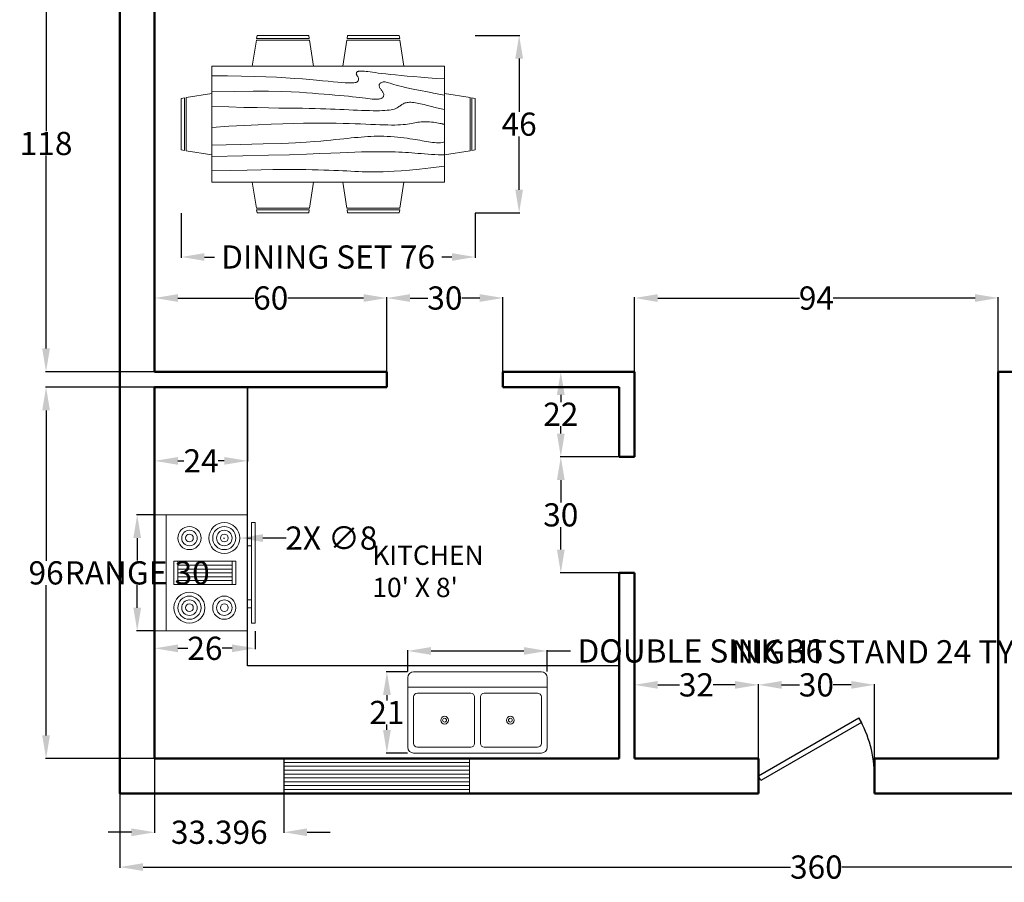
# Model space of a CAD drawing. Units: inches. Extents: x -8 to 445, y -363 to 43.
# Tile 1 of 3: x -8 to 246, y -363 to -140. Entities that reach past the tile are written whole.
import ezdxf

# ---------------------------------------------------------------- set-up
doc = ezdxf.new("R2010")
doc.units = ezdxf.units.IN
doc.header["$MEASUREMENT"] = 0
for name, color, linetype, lineweight in [('A-ANNO-DIMS', 2, 'Continuous', 18), ('A-AREA-IDEN', 7, 'Continuous', 18), ('A-EQPM', 9, 'Continuous', 18), ('A-FLOR-CASE', 9, 'Continuous', 25), ('A-FLOR-FIXT', 9, 'Continuous', 18), ('A-FURN', 8, 'Continuous', 18), ('A-WALL', 7, 'Continuous', 50), ('DOORS', 43, 'Continuous', 25), ('WINDOWS', 140, 'Continuous', 18)]:
    doc.layers.add(name, color=color, linetype=linetype, lineweight=lineweight)
doc.styles.get("Standard").update_dxf_attribs({"font": 'arial.ttf'})
doc.dimstyles.get("Standard").update_dxf_attribs({"dimtxt": 6, "dimasz": 6, "dimexe": 0.18, "dimexo": 0.0625, "dimgap": 0.09, "dimtad": 0, "dimtih": 1, "dimtoh": 1, "dimdec": 0, "dimzin": 0, "dimdsep": 46, "dimlunit": 4, "dimtxsty": 'Standard', "dimcen": 0.09, "dimadec": 0, "dimazin": 0, "dimtfac": 1, "dimtdec": 0, "dimtofl": 0, "dimtmove": 0, "dimatfit": 3, "dimfxl": 1, "dimtolj": 1, "dimtzin": 0, "dimarcsym": 0})

# ---------------------------------------------------------------- blocks, each defined once
blk = doc.blocks.new('*U2')
for p, q in [((0, 0), (0, -6)), ((40, 0), (40, -6))]:
    blk.add_line(p, q)
blk.add_lwpolyline([(0, 0), (34.64, 20), (35.52, 18.48), (0.87, -1.52)], close=True)
blk.add_arc((0, 0), 40, 0, 30)
blk = doc.blocks.new('Dining Set - 36 x 72 in.')
for p, q in [((-22, 27.5), (-22.1562, 26.50042)), ((-22, 27.5), (-6, 27.5)), ((-5.8437, 26.49966), (-6, 27.5)), ((6, 27.5), (5.8438, 26.50042)), ((6, 27.5), (22, 27.5)), ((22.1563, 26.49966), (22, 27.5)), ((-22.2343, 26.00059), (-23.4847, 17.99762)), ((-22.2304, 26), (-5.7608, 26)), ((-5.8416, 26.5), (-22.1534, 26.5)), ((-4.5152, 17.99762), (-5.7655, 25.99926)), ((5.7657, 26.00059), (4.5153, 17.99762)), ((5.7696, 26), (22.2392, 26)), ((22.1584, 26.5), (5.8466, 26.5)), ((23.4848, 17.99762), (22.2345, 25.99926)), ((36, 18), (-36, 18)), ((-36, 18), (-36, -18)), ((36, -18), (36, 18)), ((-44.0006, 8.23428), (-35.9976, 9.48474)), ((44.0006, 8.23428), (35.9976, 9.48474)), ((-45.5, 8), (-44.5004, 8.15617)), ((-45.5, 8), (-45.5, -8)), ((-44.5, -8.15843), (-44.5, 8.15338)), ((-44, 8.23041), (-44, -8.23915)), ((44, 8.23041), (44, -8.23915)), ((44.5, -8.15843), (44.5, 8.15338)), ((45.5, 8), (44.5005, 8.15617)), ((45.5, 8), (45.5, -8)), ((-44.4997, -8.15631), (-45.5, -8)), ((-35.9976, -9.48476), (-43.9993, -8.2345)), ((35.9976, -9.48476), (43.9993, -8.2345)), ((44.4997, -8.15631), (45.5, -8)), ((-36, -18), (36, -18)), ((-22.2343, -26.0006), (-23.4847, -17.99762)), ((-4.5152, -17.99762), (-5.7655, -25.99928)), ((5.7657, -26.0006), (4.5153, -17.99762)), ((23.4848, -17.99762), (22.2345, -25.99928)), ((-22.2304, -26), (-5.7608, -26)), ((-22, -27.5), (-22.1562, -26.50044)), ((-5.8416, -26.5), (-22.1534, -26.5)), ((-5.8437, -26.49967), (-6, -27.5)), ((5.7696, -26), (22.2392, -26)), ((6, -27.5), (5.8438, -26.50044)), ((22.1584, -26.5), (5.8466, -26.5)), ((22.1563, -26.49967), (22, -27.5)), ((-22, -27.5), (-6, -27.5)), ((6, -27.5), (22, -27.5))]:
    blk.add_line(p, q)
for points in [[(-36, 15), (-31.1772, 14.97754), (-26.8079, 14.91406), (-22.8538, 14.81543), (-19.276, 14.6875), (-16.0362, 14.53613), (-13.0957, 14.36718), (-10.4159, 14.18652), (-7.9583, 14), (-5.6904, 13.81315), (-3.6035, 13.63021), (-1.6954, 13.45508), (0.0365, 13.29166), (1.5945, 13.14388), (2.9811, 13.01562), (4.1988, 12.9108), (5.25, 12.83333), (6.1393, 12.78613), (6.8802, 12.76823), (7.4883, 12.77767), (7.9792, 12.8125), (8.3685, 12.87077), (8.6719, 12.95052), (8.9049, 13.0498), (9.0833, 13.16666), (9.2205, 13.29899), (9.3216, 13.44401), (9.3895, 13.59879), (9.4271, 13.76041), (9.4373, 13.92594), (9.4232, 14.09245), (9.3875, 14.257), (9.3333, 14.41666), (9.2638, 14.56917), (9.1836, 14.71484), (9.0975, 14.85465), (9.0104, 14.98958), (8.9272, 15.1206), (8.8529, 15.2487), (8.7922, 15.37483), (8.75, 15.5), (8.7305, 15.62467), (8.7344, 15.74739), (8.7617, 15.86621), (8.8125, 15.97916), (8.8867, 16.08431), (8.9844, 16.17968), (9.1055, 16.26334), (9.25, 16.33333), (9.4189, 16.38802), (9.6172, 16.42708), (9.8506, 16.45052), (10.125, 16.45833), (10.4463, 16.45052), (10.8203, 16.42708), (11.2529, 16.38802), (11.75, 16.33333), (12.3184, 16.26318), (12.9694, 16.17838), (13.7151, 16.07991), (14.5677, 15.96875), (15.5395, 15.84586), (16.6426, 15.71224), (17.8893, 15.56884), (19.2917, 15.41666), (20.859, 15.25667), (22.5879, 15.08984), (24.4721, 14.91715), (26.5052, 14.73958), (28.6809, 14.5581), (30.9929, 14.3737), (33.4347, 14.18733), (36, 14)], [(-36, 10), (-28.9766, 10.14274), (-23.1725, 10.20442), (-18.4241, 10.19775), (-14.5677, 10.13541), (-11.4399, 10.03011), (-8.877, 9.89453), (-6.7154, 9.74137), (-4.7917, 9.58333), (-2.9698, 9.43082), (-1.2246, 9.28515), (0.4415, 9.14534), (2.026, 9.01041), (3.5266, 8.87939), (4.9408, 8.7513), (6.266, 8.62516), (7.5, 8.5), (8.6411, 8.37549), (9.6914, 8.2539), (10.6538, 8.13818), (11.5312, 8.03125), (12.3267, 7.93603), (13.043, 7.85547), (13.6831, 7.79248), (14.25, 7.75), (14.7471, 7.7303), (15.1797, 7.73307), (15.5537, 7.75732), (15.875, 7.80208), (16.1494, 7.86637), (16.3828, 7.94922), (16.5811, 8.04964), (16.75, 8.16666), (16.8944, 8.29915), (17.0143, 8.44531), (17.1089, 8.60319), (17.1771, 8.77083), (17.218, 8.94629), (17.2305, 9.1276), (17.2137, 9.31282), (17.1667, 9.5), (17.0895, 9.6875), (16.987, 9.875), (16.8649, 10.0625), (16.7292, 10.25), (16.5856, 10.4375), (16.4401, 10.625), (16.2985, 10.8125), (16.1667, 11), (16.05, 11.18733), (15.9518, 11.3737), (15.8752, 11.5581), (15.8229, 11.73958), (15.798, 11.91715), (15.8034, 12.08984), (15.842, 12.25667), (15.9167, 12.41666), (16.0295, 12.56836), (16.1784, 12.70833), (16.3605, 12.83268), (16.5729, 12.9375), (16.8127, 13.01888), (17.0768, 13.07291), (17.3625, 13.0957), (17.6667, 13.08333), (17.9894, 13.03312), (18.3418, 12.94726), (18.7382, 12.82918), (19.1927, 12.68229), (19.7195, 12.51001), (20.3327, 12.31575), (21.0465, 12.10294), (21.875, 11.875), (22.8357, 11.63354), (23.959, 11.37304), (25.2786, 11.08618), (26.8282, 10.76562), (28.6414, 10.40405), (30.752, 9.99414), (33.1936, 9.52856), (36, 9)], [(-36, 5.5), (-30.7157, 5.3348), (-26.069, 5.20963), (-21.9946, 5.11767), (-18.4271, 5.05208), (-15.3009, 5.00602), (-12.5508, 4.97265), (-10.1112, 4.94515), (-7.9167, 4.91666), (-5.909, 4.88167), (-4.0586, 4.83984), (-2.3429, 4.79215), (-0.7396, 4.73958), (0.7739, 4.6831), (2.22, 4.6237), (3.6213, 4.56233), (5, 4.5), (6.373, 4.43782), (7.7344, 4.3776), (9.0723, 4.32129), (10.375, 4.27083), (11.6309, 4.22819), (12.8281, 4.19531), (13.9551, 4.17415), (15, 4.16666), (15.954, 4.17448), (16.819, 4.19791), (17.6001, 4.23698), (18.3021, 4.29166), (18.9299, 4.36198), (19.4883, 4.44791), (19.9823, 4.54948), (20.4167, 4.66666), (20.7969, 4.79899), (21.1302, 4.94401), (21.4245, 5.09879), (21.6875, 5.26041), (21.9271, 5.42594), (22.1511, 5.59245), (22.3672, 5.757), (22.5834, 5.91666), (22.8065, 6.06868), (23.0404, 6.21093), (23.2879, 6.34147), (23.5521, 6.45833), (23.8358, 6.55957), (24.142, 6.64323), (24.4735, 6.70735), (24.8334, 6.75), (25.2235, 6.76969), (25.642, 6.76692), (26.0858, 6.74267), (26.5521, 6.69791), (27.0379, 6.63362), (27.5404, 6.55078), (28.0565, 6.45036), (28.5834, 6.33333), (29.1242, 6.19987), (29.7071, 6.04687), (30.3661, 5.87044), (31.1354, 5.66666), (32.0493, 5.43164), (33.142, 5.16146), (34.4475, 4.85221), (36, 4.5)], [(-36, -1), (-30.7915, -0.6591), (-26.0195, -0.38216), (-21.6519, -0.16284), (-17.6563, 0.00521), (-14.0005, 0.12833), (-10.6523, 0.21289), (-7.5796, 0.26522), (-4.75, 0.29166), (-2.134, 0.29793), (0.2878, 0.28711), (2.5317, 0.26163), (4.6146, 0.22396), (6.5529, 0.17651), (8.3633, 0.12174), (10.0623, 0.06209), (11.6667, 0), (13.1899, -0.06201), (14.6341, -0.1211), (15.9982, -0.17432), (17.2813, -0.21875), (18.4823, -0.25147), (19.6003, -0.26953), (20.6343, -0.27002), (21.5834, -0.25), (22.4481, -0.20768), (23.2357, -0.14584), (23.9549, -0.06836), (24.6146, 0.02083), (25.2235, 0.11784), (25.7904, 0.21875), (26.3241, 0.31966), (26.8334, 0.41666), (27.3265, 0.50618), (27.8099, 0.58593), (28.2894, 0.65397), (28.7709, 0.70833), (29.2601, 0.74707), (29.763, 0.76823), (30.2855, 0.76985), (30.8334, 0.75), (31.4088, 0.70784), (31.9994, 0.64713), (32.589, 0.57275), (33.1615, 0.48958), (33.7008, 0.4025), (34.1908, 0.3164), (34.6153, 0.23616), (34.9584, 0.16666), (35.2099, 0.11165), (35.3848, 0.07031), (35.504, 0.04069), (35.5886, 0.02083), (35.6594, 0.00879), (35.7377, 0.0026), (35.8442, 0.00032), (36, 0)], [(-36, -6.5), (-27.1843, -6.31267), (-20.084, -6.1263), (-14.469, -5.9419), (-10.1094, -5.76042), (-6.7752, -5.58285), (-4.2363, -5.41016), (-2.2629, -5.24333), (-0.625, -5.08334), (0.8708, -4.93099), (2.2715, -4.78646), (3.5872, -4.64974), (4.8281, -4.52084), (6.0046, -4.39974), (7.127, -4.28646), (8.2053, -4.18099), (9.25, -4.08334), (10.2705, -3.99382), (11.2734, -3.91407), (12.2647, -3.84603), (13.25, -3.79167), (14.2354, -3.75293), (15.2266, -3.73177), (16.2295, -3.73015), (17.25, -3.75), (18.2912, -3.79248), (19.3451, -3.85547), (20.4009, -3.93604), (21.4479, -4.03125), (22.4754, -4.13819), (23.4727, -4.25391), (24.4289, -4.37549), (25.3334, -4.5), (26.1785, -4.62492), (26.9694, -4.74935), (27.7145, -4.87281), (28.4219, -4.99479), (29.1, -5.11483), (29.7572, -5.23242), (30.4016, -5.34709), (31.0417, -5.45834), (31.6837, -5.56437), (32.3262, -5.65821), (32.9658, -5.73153), (33.599, -5.77604), (34.2224, -5.78345), (34.8327, -5.74545), (35.4264, -5.65373), (36, -5.5)], [(-36, -10), (-26.4022, -9.81299), (-18.4675, -9.62891), (-11.9839, -9.45069), (-6.7396, -9.28125), (-2.5226, -9.12354), (0.8789, -8.98047), (3.6769, -8.85498), (6.0833, -8.75), (8.2767, -8.66765), (10.3021, -8.60677), (12.1712, -8.56543), (13.8958, -8.54167), (15.4876, -8.53353), (16.9583, -8.53907), (18.3197, -8.55632), (19.5834, -8.58334), (20.7616, -8.61841), (21.8685, -8.66081), (22.9188, -8.71004), (23.9271, -8.76563), (24.9081, -8.82707), (25.8763, -8.89388), (26.8465, -8.96558), (27.8334, -9.04167), (28.8474, -9.12118), (29.8828, -9.20117), (30.93, -9.27824), (31.9792, -9.34896), (33.0205, -9.40991), (34.0443, -9.45768), (35.0407, -9.48885), (36, -9.5)], [(-36, -14.5), (-30.0881, -14.33513), (-25.0332, -14.21224), (-20.7312, -14.12647), (-17.0781, -14.07292), (-13.97, -14.04671), (-11.3027, -14.04297), (-8.9724, -14.05681), (-6.875, -14.08334), (-4.9224, -14.11833), (-3.0905, -14.16016), (-1.3709, -14.20785), (0.2448, -14.26042), (1.7647, -14.3169), (3.1973, -14.3763), (4.5507, -14.43767), (5.8333, -14.5), (7.0554, -14.5621), (8.235, -14.62175), (9.3922, -14.67652), (10.5469, -14.72396), (11.7192, -14.76164), (12.929, -14.78711), (14.1965, -14.79794), (15.5417, -14.79167), (16.9933, -14.76424), (18.6152, -14.70508), (20.4804, -14.60197), (22.6615, -14.44271), (25.2312, -14.21509), (28.2624, -13.9069), (31.8277, -13.50594), (36, -13)]]:
    blk.add_lwpolyline(points)
blk = doc.blocks.new('Range-Oven - 30 in top')
for p, q in [((0, -3), (30, -3)), ((12, -6), (18, -6)), ((13, -20), (13, -6)), ((14, -6), (14, -20)), ((15, -20), (15, -6)), ((16, -6), (16, -20)), ((17, -20), (17, -6)), ((18, -20), (12, -20)), ((6, -24), (6, -25)), ((8, -25), (8, -24)), ((22, -25), (22, -24)), ((24, -24), (24, -25))]:
    blk.add_line(p, q)
for points in [[(0, -24), (0, 0), (30, 0), (30, -24)], [(12, -21), (12, -5), (18, -5), (18, -21)], [(2, -26), (2, -25), (28, -25), (28, -26)]]:
    blk.add_lwpolyline(points, close=True)
for centre, radius in [((6, -9), 4), ((6, -9), 3), ((6, -9), 2), ((24, -9), 3), ((24, -9), 2), ((6, -9), 1), ((24, -9), 1), ((6, -18), 3), ((24, -18), 4), ((24, -18), 3), ((6, -18), 2), ((6, -18), 1), ((24, -18), 2), ((24, -18), 1)]:
    blk.add_circle(centre, radius)
blk = doc.blocks.new('Sink-double - 36 in top')
for p, q in [((-18, -4), (18, -4)), ((-0.75, -18.5), (-0.75, -6.5)), ((0.75, -6.5), (0.75, -18.5))]:
    blk.add_line(p, q)
for points in [[(-16.5, 0), (16.5, 0)], [(-18, -19.5), (-18, -1.5)], [(18, -1.5), (18, -19.5)], [(-16.5, -18.5), (-16.5, -6.5)], [(-15.5, -5.5), (-1.75, -5.5)], [(1.75, -5.5), (15.5, -5.5)], [(16.5, -6.5), (16.5, -18.5)], [(-1.75, -19.5), (-15.5, -19.5)], [(15.5, -19.5), (1.75, -19.5)], [(16.5, -21), (-16.5, -21)]]:
    blk.add_lwpolyline(points)
for centre, radius in [((-8.5, -12.5), 1), ((-8.5, -12.5), 0.5), ((8.5, -12.5), 1), ((8.5, -12.5), 0.5)]:
    blk.add_circle(centre, radius)
for centre, radius, start, end in [((-16.5, -1.5), 1.5, 90, 180), ((16.5, -1.5), 1.5, 0, 90), ((-15.5, -6.5), 1, 90, 180), ((-1.75, -6.5), 1, 0, 90), ((1.75, -6.5), 1, 90, 180), ((15.5, -6.5), 1, 0, 90), ((-16.5, -19.5), 1.5, 180, 270), ((-15.5, -18.5), 1, 180, 270), ((-1.75, -18.5), 1, 270, 0), ((1.75, -18.5), 1, 180, 270), ((15.5, -18.5), 1, 270, 0), ((16.5, -19.5), 1.5, 270, 0)]:
    blk.add_arc(centre, radius, start, end)
blk = doc.blocks.new('WIN-48IN')
for p, q in [((0, 0), (0, 9)), ((0, 9), (48, 9)), ((0, 8), (48, 8)), ((48, 9), (48, 0)), ((0, 7), (48, 7)), ((0, 6), (48, 6)), ((0, 5), (48, 5)), ((0, 4), (48, 4)), ((0, 3), (48, 3)), ((0, 2), (48, 2)), ((48, 1), (0, 1)), ((48, 0), (0, 0))]:
    blk.add_line(p, q)
blk = doc.blocks.new('*D19')
at = {"layer": 'A-ANNO-DIMS', "color": 0, "lineweight": -2, "transparency": 16777216}
for p, q in [((265.09, -303.49), (259.09, -303.49)), ((265.09, -307.03), (265.09, -303.31)), ((283.09, -303.49), (271.09, -303.49)), ((289.09, -307.03), (289.09, -303.31))]:
    blk.add_line(p, q, dxfattribs=at)
at = {"layer": 'A-ANNO-DIMS', "color": 0, "transparency": 16777216}
for points in [[(271.09, -302.49), (271.09, -304.49), (265.09, -303.49)], [(283.09, -302.49), (283.09, -304.49), (289.09, -303.49)]]:
    blk.add_solid(points, dxfattribs=at)
at = {"layer": 'Defpoints', "color": 0, "transparency": 16777216}
for p in [(265.09, -303.49), (265.09, -307.09), (289.09, -307.09)]:
    blk.add_point(p, dxfattribs=at)
at = {"layer": 'A-ANNO-DIMS', "color": 0, "transparency": 16777216, "insert": (216.13, -303.49), "char_height": 6, "attachment_point": 5}
blk.add_mtext('\\A1;NIGHTSTAND 24 TYP.', dxfattribs=at)
blk = doc.blocks.new('*D27')
at = {"layer": 'A-ANNO-DIMS', "color": 0, "lineweight": -2, "transparency": 16777216}
for p, q in [((33.76, -190.11), (33.76, -201.62)), ((109.69, -190.11), (109.69, -201.62)), ((39.76, -201.44), (42.34, -201.44)), ((103.69, -201.44), (101.11, -201.44))]:
    blk.add_line(p, q, dxfattribs=at)
at = {"layer": 'A-ANNO-DIMS', "color": 0, "transparency": 16777216}
for points in [[(39.76, -200.44), (39.76, -202.44), (33.76, -201.44)], [(103.69, -200.44), (103.69, -202.44), (109.69, -201.44)]]:
    blk.add_solid(points, dxfattribs=at)
at = {"layer": 'Defpoints', "color": 0, "transparency": 16777216}
for p in [(33.76, -190.05), (109.69, -190.05), (109.69, -201.44)]:
    blk.add_point(p, dxfattribs=at)
at = {"layer": 'A-ANNO-DIMS', "color": 0, "transparency": 16777216, "insert": (71.72, -201.44), "char_height": 6, "attachment_point": 5}
blk.add_mtext('\\A1;DINING SET 76', dxfattribs=at)
blk = doc.blocks.new('*D28')
at = {"layer": 'A-ANNO-DIMS', "color": 0, "lineweight": -2, "transparency": 16777216}
for p, q in [((109.75, -144.15), (121.26, -144.15)), ((121.08, -150.15), (121.08, -163.95)), ((121.08, -184.05), (121.08, -170.25)), ((109.75, -190.05), (121.26, -190.05))]:
    blk.add_line(p, q, dxfattribs=at)
at = {"layer": 'A-ANNO-DIMS', "color": 0, "transparency": 16777216}
for points in [[(120.08, -150.15), (122.08, -150.15), (121.08, -144.15)], [(120.08, -184.05), (122.08, -184.05), (121.08, -190.05)]]:
    blk.add_solid(points, dxfattribs=at)
at = {"layer": 'Defpoints', "color": 0, "transparency": 16777216}
for p in [(109.69, -144.15), (121.08, -144.15), (109.69, -190.05)]:
    blk.add_point(p, dxfattribs=at)
at = {"layer": 'A-ANNO-DIMS', "color": 0, "transparency": 16777216, "insert": (121.08, -167.1), "char_height": 6, "attachment_point": 5}
blk.add_mtext('\\A1;46', dxfattribs=at)
blk = doc.blocks.new('*D29')
at = {"layer": 'A-ANNO-DIMS', "color": 0, "lineweight": -2, "transparency": 16777216}
for p, q in [((26.82, -268.09), (22.21, -268.09)), ((22.39, -274.09), (22.39, -279.9)), ((22.39, -292.09), (22.39, -286.29)), ((26.82, -298.09), (22.21, -298.09))]:
    blk.add_line(p, q, dxfattribs=at)
at = {"layer": 'A-ANNO-DIMS', "color": 0, "transparency": 16777216}
for points in [[(21.39, -274.09), (23.39, -274.09), (22.39, -268.09)], [(21.39, -292.09), (23.39, -292.09), (22.39, -298.09)]]:
    blk.add_solid(points, dxfattribs=at)
at = {"layer": 'Defpoints', "color": 0, "transparency": 16777216}
for p in [(22.39, -268.09), (26.89, -268.09), (26.89, -298.09)]:
    blk.add_point(p, dxfattribs=at)
at = {"layer": 'A-ANNO-DIMS', "color": 0, "transparency": 16777216, "insert": (22.39, -283.09), "char_height": 6, "attachment_point": 5}
blk.add_mtext('\\A1;RANGE 30', dxfattribs=at)
blk = doc.blocks.new('*D30')
at = {"layer": 'A-ANNO-DIMS', "color": 0, "lineweight": -2, "transparency": 16777216}
for p, q in [((26.89, -298.15), (26.89, -302.77)), ((52.89, -298.15), (52.89, -302.77)), ((32.89, -302.59), (35.45, -302.59)), ((46.89, -302.59), (44.32, -302.59))]:
    blk.add_line(p, q, dxfattribs=at)
at = {"layer": 'A-ANNO-DIMS', "color": 0, "transparency": 16777216}
for points in [[(32.89, -301.59), (32.89, -303.59), (26.89, -302.59)], [(46.89, -301.59), (46.89, -303.59), (52.89, -302.59)]]:
    blk.add_solid(points, dxfattribs=at)
at = {"layer": 'Defpoints', "color": 0, "transparency": 16777216}
for p in [(26.89, -298.09), (52.89, -298.09), (26.89, -302.59)]:
    blk.add_point(p, dxfattribs=at)
at = {"layer": 'A-ANNO-DIMS', "color": 0, "transparency": 16777216, "insert": (39.89, -302.59), "char_height": 6, "attachment_point": 5}
blk.add_mtext('\\A1;26', dxfattribs=at)
blk = doc.blocks.new('*D31')
at = {"layer": 'A-ANNO-DIMS', "color": 0, "lineweight": -2, "transparency": 16777216}
for p, q in [((92.31, -308.61), (92.31, -303.09)), ((98.31, -303.27), (122.31, -303.27)), ((128.31, -308.61), (128.31, -303.09)), ((128.31, -303.27), (134.31, -303.27))]:
    blk.add_line(p, q, dxfattribs=at)
at = {"layer": 'A-ANNO-DIMS', "color": 0, "transparency": 16777216}
for points in [[(98.31, -302.27), (98.31, -304.27), (92.31, -303.27)], [(122.31, -302.27), (122.31, -304.27), (128.31, -303.27)]]:
    blk.add_solid(points, dxfattribs=at)
at = {"layer": 'Defpoints', "color": 0, "transparency": 16777216}
for p in [(128.31, -303.27), (92.31, -308.67), (128.31, -308.67)]:
    blk.add_point(p, dxfattribs=at)
at = {"layer": 'A-ANNO-DIMS', "color": 0, "transparency": 16777216, "insert": (167.89, -303.27), "char_height": 6, "attachment_point": 5}
blk.add_mtext('\\A1;DOUBLE SINK 36', dxfattribs=at)
blk = doc.blocks.new('*D32')
at = {"layer": 'A-ANNO-DIMS', "color": 0, "lineweight": -2, "transparency": 16777216}
for p, q in [((92.25, -308.67), (86.73, -308.67)), ((86.91, -314.67), (86.91, -316.07)), ((86.91, -323.67), (86.91, -322.27)), ((92.25, -329.67), (86.73, -329.67))]:
    blk.add_line(p, q, dxfattribs=at)
at = {"layer": 'A-ANNO-DIMS', "color": 0, "transparency": 16777216}
for points in [[(85.91, -314.67), (87.91, -314.67), (86.91, -308.67)], [(85.91, -323.67), (87.91, -323.67), (86.91, -329.67)]]:
    blk.add_solid(points, dxfattribs=at)
at = {"layer": 'Defpoints', "color": 0, "transparency": 16777216}
for p in [(86.91, -308.67), (92.31, -308.67), (92.31, -329.67)]:
    blk.add_point(p, dxfattribs=at)
at = {"layer": 'A-ANNO-DIMS', "color": 0, "transparency": 16777216, "insert": (86.91, -319.17), "char_height": 6, "attachment_point": 5}
blk.add_mtext('\\A1;21', dxfattribs=at)
blk = doc.blocks.new('*D33')
at = {"layer": 'A-ANNO-DIMS', "color": 0, "lineweight": -2, "transparency": 16777216}
for p, q in [((17.89, -340.15), (17.89, -359.32)), ((377.89, -340.15), (377.89, -359.32)), ((23.89, -359.14), (191.18, -359.14)), ((371.89, -359.14), (204.59, -359.14))]:
    blk.add_line(p, q, dxfattribs=at)
at = {"layer": 'A-ANNO-DIMS', "color": 0, "transparency": 16777216}
for points in [[(23.89, -358.14), (23.89, -360.14), (17.89, -359.14)], [(371.89, -358.14), (371.89, -360.14), (377.89, -359.14)]]:
    blk.add_solid(points, dxfattribs=at)
at = {"layer": 'Defpoints', "color": 0, "transparency": 16777216}
for p in [(17.89, -340.09), (377.89, -340.09), (377.89, -359.14)]:
    blk.add_point(p, dxfattribs=at)
at = {"layer": 'A-ANNO-DIMS', "color": 0, "transparency": 16777216, "insert": (197.89, -359.14), "char_height": 6, "attachment_point": 5}
blk.add_mtext('\\A1;360', dxfattribs=at)
blk = doc.blocks.new('*D41')
at = {"layer": 'A-ANNO-DIMS', "color": 0, "lineweight": -2, "transparency": 16777216}
for p, q in [((26.82, -113.09), (-1.34, -113.09)), ((-1.16, -119.09), (-1.16, -168.94)), ((-1.16, -225.09), (-1.16, -175.24)), ((26.82, -231.09), (-1.34, -231.09))]:
    blk.add_line(p, q, dxfattribs=at)
at = {"layer": 'A-ANNO-DIMS', "color": 0, "transparency": 16777216}
for points in [[(-2.16, -119.09), (-0.16, -119.09), (-1.16, -113.09)], [(-2.16, -225.09), (-0.16, -225.09), (-1.16, -231.09)]]:
    blk.add_solid(points, dxfattribs=at)
at = {"layer": 'Defpoints', "color": 0, "transparency": 16777216}
for p in [(-1.16, -113.09), (26.89, -113.09), (26.89, -231.09)]:
    blk.add_point(p, dxfattribs=at)
at = {"layer": 'A-ANNO-DIMS', "color": 0, "transparency": 16777216, "insert": (-1.16, -172.09), "char_height": 6, "attachment_point": 5}
blk.add_mtext('\\A1;118', dxfattribs=at)
blk = doc.blocks.new('*D42')
at = {"layer": 'A-ANNO-DIMS', "color": 0, "lineweight": -2, "transparency": 16777216}
for p, q in [((26.82, -235.09), (-1.34, -235.09)), ((-1.16, -241.09), (-1.16, -279.94)), ((-1.16, -325.09), (-1.16, -286.24)), ((26.82, -331.09), (-1.34, -331.09))]:
    blk.add_line(p, q, dxfattribs=at)
at = {"layer": 'A-ANNO-DIMS', "color": 0, "transparency": 16777216}
for points in [[(-2.16, -241.09), (-0.16, -241.09), (-1.16, -235.09)], [(-2.16, -325.09), (-0.16, -325.09), (-1.16, -331.09)]]:
    blk.add_solid(points, dxfattribs=at)
at = {"layer": 'Defpoints', "color": 0, "transparency": 16777216}
for p in [(-1.16, -235.09), (26.89, -235.09), (26.89, -331.09)]:
    blk.add_point(p, dxfattribs=at)
at = {"layer": 'A-ANNO-DIMS', "color": 0, "transparency": 16777216, "insert": (-1.16, -283.09), "char_height": 6, "attachment_point": 5}
blk.add_mtext('\\A1;96', dxfattribs=at)
blk = doc.blocks.new('*D43')
at = {"layer": 'A-ANNO-DIMS', "color": 0, "lineweight": -2, "transparency": 16777216}
for p, q in [((182.89, -331.03), (182.89, -311.86)), ((188.89, -312.04), (193.51, -312.04)), ((206.89, -312.04), (202.26, -312.04)), ((212.89, -331.03), (212.89, -311.86))]:
    blk.add_line(p, q, dxfattribs=at)
at = {"layer": 'A-ANNO-DIMS', "color": 0, "transparency": 16777216}
for points in [[(188.89, -311.04), (188.89, -313.04), (182.89, -312.04)], [(206.89, -311.04), (206.89, -313.04), (212.89, -312.04)]]:
    blk.add_solid(points, dxfattribs=at)
at = {"layer": 'Defpoints', "color": 0, "transparency": 16777216}
for p in [(212.89, -312.04), (182.89, -331.09), (212.89, -331.09)]:
    blk.add_point(p, dxfattribs=at)
at = {"layer": 'A-ANNO-DIMS', "color": 0, "transparency": 16777216, "insert": (197.89, -312.04), "char_height": 6, "attachment_point": 5}
blk.add_mtext('\\A1;30', dxfattribs=at)
blk = doc.blocks.new('*D44')
at = {"layer": 'A-ANNO-DIMS', "color": 0, "lineweight": -2, "transparency": 16777216}
for p, q in [((150.89, -331.03), (150.89, -311.86)), ((156.89, -312.04), (162.53, -312.04)), ((176.89, -312.04), (171.24, -312.04)), ((182.89, -331.03), (182.89, -311.86))]:
    blk.add_line(p, q, dxfattribs=at)
at = {"layer": 'A-ANNO-DIMS', "color": 0, "transparency": 16777216}
for points in [[(156.89, -311.04), (156.89, -313.04), (150.89, -312.04)], [(176.89, -311.04), (176.89, -313.04), (182.89, -312.04)]]:
    blk.add_solid(points, dxfattribs=at)
at = {"layer": 'Defpoints', "color": 0, "transparency": 16777216}
for p in [(182.89, -312.04), (150.89, -331.09), (182.89, -331.09)]:
    blk.add_point(p, dxfattribs=at)
at = {"layer": 'A-ANNO-DIMS', "color": 0, "transparency": 16777216, "insert": (166.89, -312.04), "char_height": 6, "attachment_point": 5}
blk.add_mtext('\\A1;32', dxfattribs=at)
blk = doc.blocks.new('*D46')
at = {"layer": 'A-ANNO-DIMS', "color": 0, "lineweight": -2, "transparency": 16777216}
for p, q in [((26.89, -231.03), (26.89, -211.86)), ((32.89, -212.04), (52.49, -212.04)), ((80.89, -212.04), (61.28, -212.04)), ((86.89, -231.03), (86.89, -211.86))]:
    blk.add_line(p, q, dxfattribs=at)
at = {"layer": 'A-ANNO-DIMS', "color": 0, "transparency": 16777216}
for points in [[(32.89, -211.04), (32.89, -213.04), (26.89, -212.04)], [(80.89, -211.04), (80.89, -213.04), (86.89, -212.04)]]:
    blk.add_solid(points, dxfattribs=at)
at = {"layer": 'Defpoints', "color": 0, "transparency": 16777216}
for p in [(86.89, -212.04), (26.89, -231.09), (86.89, -231.09)]:
    blk.add_point(p, dxfattribs=at)
at = {"layer": 'A-ANNO-DIMS', "color": 0, "transparency": 16777216, "insert": (56.89, -212.04), "char_height": 6, "attachment_point": 5}
blk.add_mtext('\\A1;60', dxfattribs=at)
blk = doc.blocks.new('*D47')
at = {"layer": 'A-ANNO-DIMS', "color": 0, "lineweight": -2, "transparency": 16777216}
for p, q in [((86.89, -231.03), (86.89, -211.86)), ((92.89, -212.04), (97.51, -212.04)), ((110.89, -212.04), (106.26, -212.04)), ((116.89, -231.03), (116.89, -211.86))]:
    blk.add_line(p, q, dxfattribs=at)
at = {"layer": 'A-ANNO-DIMS', "color": 0, "transparency": 16777216}
for points in [[(92.89, -211.04), (92.89, -213.04), (86.89, -212.04)], [(110.89, -211.04), (110.89, -213.04), (116.89, -212.04)]]:
    blk.add_solid(points, dxfattribs=at)
at = {"layer": 'Defpoints', "color": 0, "transparency": 16777216}
for p in [(116.89, -212.04), (86.89, -231.09), (116.89, -231.09)]:
    blk.add_point(p, dxfattribs=at)
at = {"layer": 'A-ANNO-DIMS', "color": 0, "transparency": 16777216, "insert": (101.89, -212.04), "char_height": 6, "attachment_point": 5}
blk.add_mtext('\\A1;30', dxfattribs=at)
blk = doc.blocks.new('*D48')
at = {"layer": 'A-ANNO-DIMS', "color": 0, "lineweight": -2, "transparency": 16777216}
for p, q in [((150.82, -253.09), (131.66, -253.09)), ((131.84, -259.09), (131.84, -264.94)), ((131.84, -277.09), (131.84, -271.25)), ((150.82, -283.09), (131.66, -283.09))]:
    blk.add_line(p, q, dxfattribs=at)
at = {"layer": 'A-ANNO-DIMS', "color": 0, "transparency": 16777216}
for points in [[(130.84, -259.09), (132.84, -259.09), (131.84, -253.09)], [(130.84, -277.09), (132.84, -277.09), (131.84, -283.09)]]:
    blk.add_solid(points, dxfattribs=at)
at = {"layer": 'Defpoints', "color": 0, "transparency": 16777216}
for p in [(131.84, -253.09), (150.89, -253.09), (150.89, -283.09)]:
    blk.add_point(p, dxfattribs=at)
at = {"layer": 'A-ANNO-DIMS', "color": 0, "transparency": 16777216, "insert": (131.84, -268.09), "char_height": 6, "attachment_point": 5}
blk.add_mtext('\\A1;30', dxfattribs=at)
blk = doc.blocks.new('*D49')
at = {"layer": 'A-ANNO-DIMS', "color": 0, "lineweight": -2, "transparency": 16777216}
for p, q in [((150.82, -231.09), (131.66, -231.09)), ((131.84, -237.09), (131.84, -238.99)), ((131.84, -247.09), (131.84, -245.19)), ((150.82, -253.09), (131.66, -253.09))]:
    blk.add_line(p, q, dxfattribs=at)
at = {"layer": 'A-ANNO-DIMS', "color": 0, "transparency": 16777216}
for points in [[(130.84, -237.09), (132.84, -237.09), (131.84, -231.09)], [(130.84, -247.09), (132.84, -247.09), (131.84, -253.09)]]:
    blk.add_solid(points, dxfattribs=at)
at = {"layer": 'Defpoints', "color": 0, "transparency": 16777216}
for p in [(131.84, -231.09), (150.89, -231.09), (150.89, -253.09)]:
    blk.add_point(p, dxfattribs=at)
at = {"layer": 'A-ANNO-DIMS', "color": 0, "transparency": 16777216, "insert": (131.84, -242.09), "char_height": 6, "attachment_point": 5}
blk.add_mtext('\\A1;22', dxfattribs=at)
blk = doc.blocks.new('*D57')
at = {"layer": 'A-ANNO-DIMS', "color": 0, "lineweight": -2, "transparency": 16777216}
for p, q in [((150.89, -231.03), (150.89, -211.86)), ((156.89, -212.04), (193.51, -212.04)), ((238.89, -212.04), (202.26, -212.04)), ((244.89, -231.03), (244.89, -211.86))]:
    blk.add_line(p, q, dxfattribs=at)
at = {"layer": 'A-ANNO-DIMS', "color": 0, "transparency": 16777216}
for points in [[(156.89, -211.04), (156.89, -213.04), (150.89, -212.04)], [(238.89, -211.04), (238.89, -213.04), (244.89, -212.04)]]:
    blk.add_solid(points, dxfattribs=at)
at = {"layer": 'Defpoints', "color": 0, "transparency": 16777216}
for p in [(244.89, -212.04), (150.89, -231.09), (244.89, -231.09)]:
    blk.add_point(p, dxfattribs=at)
at = {"layer": 'A-ANNO-DIMS', "color": 0, "transparency": 16777216, "insert": (197.89, -212.04), "char_height": 6, "attachment_point": 5}
blk.add_mtext('\\A1;94', dxfattribs=at)
blk = doc.blocks.new('*D58')
at = {"layer": 'A-ANNO-DIMS', "color": 0, "lineweight": -2, "transparency": 16777216}
for p, q in [((26.89, -331.15), (26.89, -350.32)), ((60.28, -331.15), (60.28, -350.32)), ((20.89, -350.14), (14.89, -350.14)), ((66.28, -350.14), (72.28, -350.14))]:
    blk.add_line(p, q, dxfattribs=at)
at = {"layer": 'A-ANNO-DIMS', "color": 0, "transparency": 16777216}
for points in [[(20.89, -349.14), (20.89, -351.14), (26.89, -350.14)], [(66.28, -349.14), (66.28, -351.14), (60.28, -350.14)]]:
    blk.add_solid(points, dxfattribs=at)
at = {"layer": 'Defpoints', "color": 0, "transparency": 16777216}
for p in [(26.89, -331.09), (60.28, -331.09), (26.89, -350.14)]:
    blk.add_point(p, dxfattribs=at)
at = {"layer": 'A-ANNO-DIMS', "color": 0, "transparency": 16777216, "insert": (43.59, -350.14), "char_height": 6, "attachment_point": 5}
blk.add_mtext('\\A1;33.396', dxfattribs=at)
blk = doc.blocks.new('*D60')
at = {"layer": 'A-ANNO-DIMS', "color": 0, "lineweight": -2, "transparency": 16777216}
for p, q in [((26.89, -235.15), (26.89, -254.32)), ((50.89, -235.15), (50.89, -254.32)), ((32.89, -254.14), (34.46, -254.14)), ((44.89, -254.14), (43.31, -254.14))]:
    blk.add_line(p, q, dxfattribs=at)
at = {"layer": 'A-ANNO-DIMS', "color": 0, "transparency": 16777216}
for points in [[(32.89, -253.14), (32.89, -255.14), (26.89, -254.14)], [(44.89, -253.14), (44.89, -255.14), (50.89, -254.14)]]:
    blk.add_solid(points, dxfattribs=at)
at = {"layer": 'Defpoints', "color": 0, "transparency": 16777216}
for p in [(26.89, -235.09), (50.89, -235.09), (26.89, -254.14)]:
    blk.add_point(p, dxfattribs=at)
at = {"layer": 'A-ANNO-DIMS', "color": 0, "transparency": 16777216, "insert": (38.89, -254.14), "char_height": 6, "attachment_point": 5}
blk.add_mtext('\\A1;24', dxfattribs=at)
blk = doc.blocks.new('*D66')
at = {"layer": 'A-ANNO-DIMS', "color": 0, "lineweight": -2, "transparency": 16777216}
for p, q in [((44.8, -274.09), (44.98, -274.09)), ((44.89, -274.18), (44.89, -274)), ((60.89, -274.09), (54.89, -274.09))]:
    blk.add_line(p, q, dxfattribs=at)
at = {"layer": 'A-ANNO-DIMS', "color": 0, "transparency": 16777216}
blk.add_solid([(54.89, -273.09), (54.89, -275.09), (48.89, -274.09)], dxfattribs=at)
at = {"layer": 'Defpoints', "color": 0, "transparency": 16777216}
for p in [(40.89, -274.09), (48.89, -274.09)]:
    blk.add_point(p, dxfattribs=at)
at = {"layer": 'A-ANNO-DIMS', "color": 0, "transparency": 16777216, "insert": (72.55, -274.09), "char_height": 6, "attachment_point": 5}
blk.add_mtext('\\A1;2X ∅8', dxfattribs=at)

msp = doc.modelspace()

# ---------------------------------------------------------------- linework, layer by layer
at = {"layer": 'A-FLOR-CASE'}
for p, q in [((50.8872, -307.0907), (50.8872, -235.0907)), ((146.8872, -307.0907), (50.8872, -307.0907))]:
    msp.add_line(p, q, dxfattribs=at)
at = {"layer": 'A-WALL'}
for p, q in [((26.8872, -231.0907), (26.8872, -113.0907)), ((86.8872, -231.0907), (26.8872, -231.0907)), ((86.8872, -235.0907), (86.8872, -231.0907)), ((150.8872, -231.0907), (116.8872, -231.0907)), ((116.8872, -235.0907), (116.8872, -231.0907)), ((150.8872, -253.0907), (150.8872, -231.0907)), ((244.8872, -231.0907), (244.8872, -331.0907)), ((254.8872, -231.0907), (244.8872, -231.0907)), ((26.8872, -331.0907), (26.8872, -235.0907)), ((86.8872, -235.0907), (26.8872, -235.0907)), ((146.8872, -235.0907), (116.8872, -235.0907)), ((146.8872, -253.0907), (146.8872, -235.0907)), ((146.8872, -253.0907), (150.8872, -253.0907)), ((146.8872, -331.0907), (146.8872, -283.0907)), ((146.8872, -283.0907), (150.8872, -283.0907)), ((150.8872, -331.0907), (150.8872, -283.0907)), ((146.8872, -331.0907), (26.8872, -331.0907)), ((182.8872, -331.0907), (150.8872, -331.0907)), ((182.8872, -331.0907), (182.8872, -340.0907)), ((244.8872, -331.0907), (212.8872, -331.0907)), ((212.8872, -331.0907), (212.8872, -340.0907))]:
    msp.add_line(p, q, dxfattribs=at)
msp.add_lwpolyline([(182.8872, -340.0907), (17.8872, -340.0907), (17.8872, 19.9093), (377.8872, 19.9093), (377.8872, -340.0907), (212.8872, -340.0907)], dxfattribs=at)

# ---------------------------------------------------------------- block references
at = {"layer": 'A-EQPM', "rotation": 89.99999999999999}
msp.add_blockref('Range-Oven - 30 in top', (26.8872, -298.0907), dxfattribs=at)
at = {"layer": 'A-FLOR-FIXT'}
msp.add_blockref('Sink-double - 36 in top', (110.3133, -308.6697), dxfattribs=at)
at = {"layer": 'A-FURN', "xscale": 0.8344141179546026, "yscale": 0.8344141179546026, "zscale": 0.8344141179546026}
msp.add_blockref('Dining Set - 36 x 72 in.', (71.7242, -167.101), dxfattribs=at)
at = {"layer": 'DOORS', "xscale": 0.75, "yscale": 0.75, "zscale": 0.75}
msp.add_blockref('*U2', (182.8872, -335.5907), dxfattribs=at)
at = {"layer": 'WINDOWS'}
msp.add_blockref('WIN-48IN', (60.2834, -340.091), dxfattribs=at)

# ---------------------------------------------------------------- texts
at = {"layer": 'A-AREA-IDEN', "insert": (83.1402, -276.0185), "char_height": 5, "attachment_point": 1}
msp.add_mtext_dynamic_manual_height_columns("KITCHEN\\P10' X 8'", width=91.815497, gutter_width=1, heights=[0], dxfattribs=at)

# ---------------------------------------------------------------- dimensions: what is measured, and where the dimension line sits
at = {"layer": 'A-ANNO-DIMS'}
for base, p1, p2, angle, override, picture, middle in [((-1.1628, -113.0907), (26.8872, -231.0907), (26.8872, -113.0907), 90, {"dimdec": 0, "dimlfac": 1, "dimrnd": 0, "dimzin": 0, "dimdsep": 46, "dimlunit": 2}, '*D41', (-1.1628, -172.0907)), ((121.0798, -144.1547), (109.69, -190.0474), (109.69, -144.1547), 90, {"dimdec": 0, "dimlfac": 1, "dimrnd": 0, "dimzin": 0, "dimdsep": 46, "dimlunit": 2}, '*D28', (121.0798, -167.101)), ((131.8372, -231.0907), (150.8872, -253.0907), (150.8872, -231.0907), 90, {"dimdec": 0, "dimlfac": 1, "dimrnd": 0, "dimzin": 0, "dimdsep": 46, "dimlunit": 2}, '*D49', (131.8372, -242.0907)), ((-1.1628, -235.0907), (26.8872, -331.0907), (26.8872, -235.0907), 90, {"dimdec": 0, "dimlfac": 1, "dimrnd": 0, "dimzin": 0, "dimdsep": 46, "dimlunit": 2}, '*D42', (-1.1628, -283.0907)), ((26.8872, -254.1407), (50.8872, -235.0907), (26.8872, -235.0907), 180, {"dimdec": 0, "dimlfac": 1, "dimrnd": 0, "dimzin": 0, "dimdsep": 46, "dimlunit": 2}, '*D60', (38.8872, -254.1407)), ((131.8372, -253.0907), (150.8872, -283.0907), (150.8872, -253.0907), 90, {"dimdec": 0, "dimlfac": 1, "dimrnd": 0, "dimzin": 0, "dimdsep": 46, "dimlunit": 2}, '*D48', (131.8372, -268.0907)), ((26.8872, -302.5907), (52.8872, -298.0907), (26.8872, -298.0907), 180, {"dimdec": 0, "dimlfac": 1, "dimrnd": 0, "dimzin": 0, "dimdsep": 46, "dimlunit": 2}, '*D30', (39.8872, -302.5907)), ((86.9133, -308.6697), (92.3133, -329.6697), (92.3133, -308.6697), 90, {"dimdec": 0, "dimlfac": 1, "dimrnd": 0, "dimzin": 0, "dimdsep": 46, "dimlunit": 2}, '*D32', (86.9133, -319.1697)), ((182.8872, -312.0407), (150.8872, -331.0907), (182.8872, -331.0907), 0, {"dimdec": 0, "dimlfac": 1, "dimrnd": 0, "dimzin": 0, "dimdsep": 46, "dimlunit": 2}, '*D44', (166.8872, -312.0407)), ((26.88724, -350.14069), (60.28368, -331.09069), (26.88724, -331.09069), 180, {"dimdec": 3, "dimlfac": 1, "dimrnd": 0, "dimzin": 0, "dimdsep": 46, "dimlunit": 2}, '*D58', (43.58546, -350.14069))]:
    dim = msp.add_linear_dim(base=base, p1=p1, p2=p2, angle=angle, dimstyle='Standard', override=override, dxfattribs=at)
    dim.commit()
    dim.dimension.update_dxf_attribs({"geometry": picture, "text_midpoint": middle})
for base, p1, p2, text, picture, middle in [((109.69, -201.4372), (33.7583, -190.0474), (109.69, -190.0474), 'DINING SET <>', '*D27', (71.7242, -201.4372)), ((128.3133, -303.2697), (92.3133, -308.6697), (128.3133, -308.6697), 'DOUBLE SINK <>', '*D31', (167.8944, -303.2697))]:
    dim = msp.add_linear_dim(base=base, p1=p1, p2=p2, text=text, dimstyle='Standard', override={"dimdec": 0, "dimlfac": 1, "dimrnd": 0, "dimzin": 0, "dimdsep": 46, "dimlunit": 2}, dxfattribs=at)
    dim.commit()
    dim.dimension.update_dxf_attribs({"geometry": picture, "text_midpoint": middle})
for base, p1, p2, picture, middle in [((86.8872, -212.0407), (26.8872, -231.0907), (86.8872, -231.0907), '*D46', (56.8872, -212.0407)), ((116.8872, -212.0407), (86.8872, -231.0907), (116.8872, -231.0907), '*D47', (101.8872, -212.0407)), ((244.8872, -212.0407), (150.8872, -231.0907), (244.8872, -231.0907), '*D57', (197.8872, -212.0407)), ((212.8872, -312.0407), (182.8872, -331.0907), (212.8872, -331.0907), '*D43', (197.8872, -312.0407)), ((377.8872, -359.1407), (17.8872, -340.0907), (377.8872, -340.0907), '*D33', (197.8872, -359.1407))]:
    dim = msp.add_linear_dim(base=base, p1=p1, p2=p2, dimstyle='Standard', override={"dimdec": 0, "dimlfac": 1, "dimrnd": 0, "dimzin": 0, "dimdsep": 46, "dimlunit": 2}, dxfattribs=at)
    dim.commit()
    dim.dimension.update_dxf_attribs({"geometry": picture, "text_midpoint": middle})
dim = msp.add_diameter_dim_2p(p1=(40.8872, -274.0904), p2=(48.8872, -274.091), text='2X <>', dimstyle='Standard', override={"dimdec": 0, "dimlfac": 1, "dimrnd": 0, "dimzin": 0, "dimdsep": 46, "dimlunit": 2}, dxfattribs=at)
dim.commit()
dim.dimension.update_dxf_attribs({"geometry": '*D66', "text_midpoint": (60.8872, -274.0919), "dimtype": 163})
for base, p1, p2, angle, text, picture, middle in [((22.3872, -268.0907), (26.8872, -298.0907), (26.8872, -268.0907), 90, 'RANGE <>', '*D29', (22.3872, -283.0907)), ((265.0866, -303.4907), (289.0866, -307.0907), (265.0866, -307.0907), 180, 'NIGHTSTAND <> TYP.', '*D19', (216.133, -303.4907))]:
    dim = msp.add_linear_dim(base=base, p1=p1, p2=p2, angle=angle, text=text, dimstyle='Standard', override={"dimdec": 0, "dimlfac": 1, "dimrnd": 0, "dimzin": 0, "dimdsep": 46, "dimlunit": 2}, dxfattribs=at)
    dim.commit()
    dim.dimension.update_dxf_attribs({"geometry": picture, "text_midpoint": middle})

doc.saveas('drawing.dxf')
